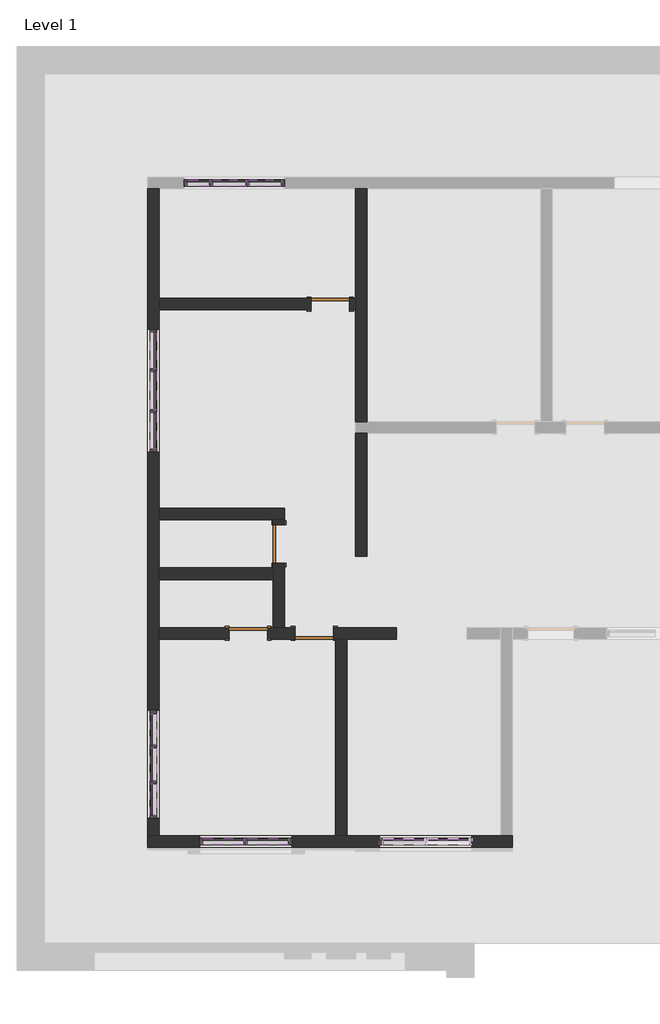
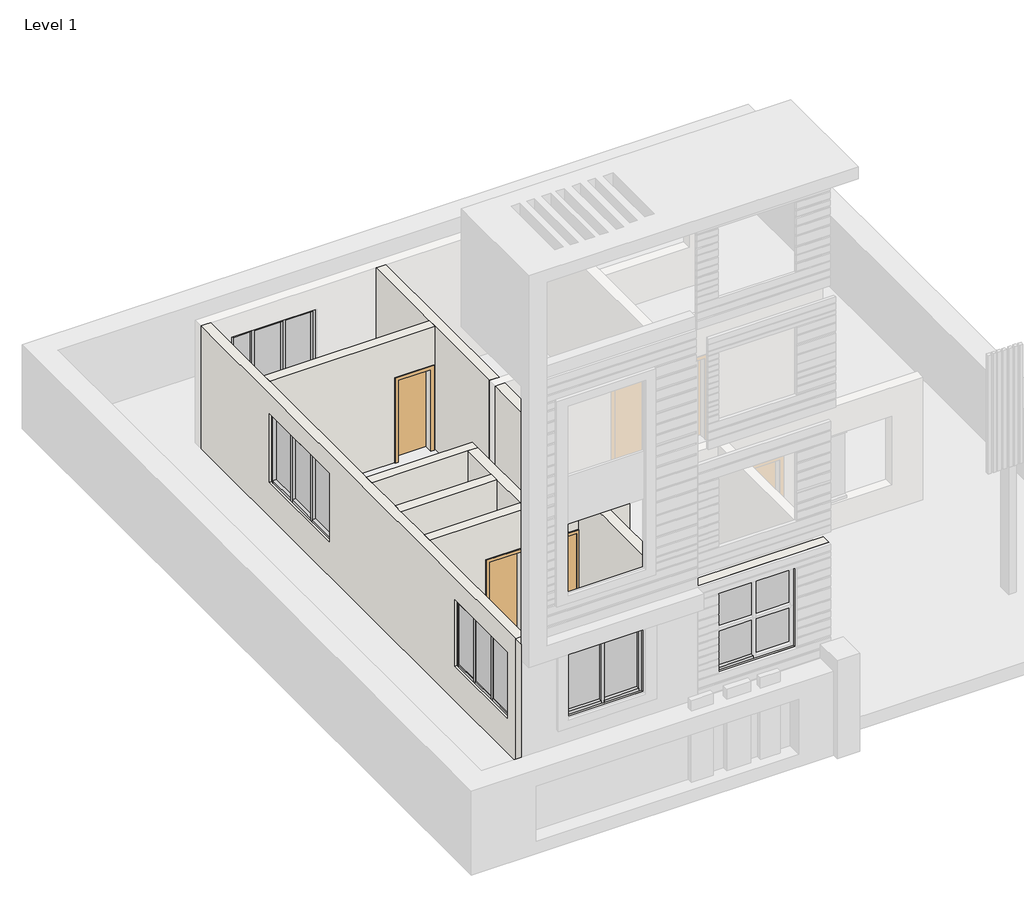
# One storey, part 1 of 2: 40 members, 15 plates, 10 walls, 4 doors.
"""IFC4 building model written with IfcOpenShell, lengths in millimetres."""

from ifc_helpers import new_model, si_unit, frame, origin, origin_with_axes, place, context, project, spatial, polyline, outline, extrude, faceted_brep, transform, mapped, element, save
from components import door_a1484949, door_85036156, member_3f0e0172, member_5215b92c, member_9d02be77, member_7007ad49, member_6fb4a552, member_d3852687, member_e7529cf5, member_eb14d2b7, member_dad99500, member_6c7e385d, member_4ab5fd4c, member_e2451291, member_36da3e1e, member_c17f1be2, member_e156fde9, member_8182dde8, member_6e7b816b, system_panel_glazed_5472c3c5, system_panel_glazed_33375d59, system_panel_glazed_3037aa96, system_panel_glazed_1cc22cd7, system_panel_glazed_f84acb07, system_panel_glazed_c72e3a3f, system_panel_glazed_c581bff3, system_panel_glazed_dab0583a, system_panel_glazed_6e362244

model = new_model("IFC4")

# Units and contexts
model_context = context("Model", 3, world=origin())
ifc_project = project(units=[si_unit("LENGTHUNIT", "METRE", prefix="MILLI")], contexts=[model_context])

# Site, building, storey
site = spatial("IfcSite", under=ifc_project)
building = spatial("IfcBuilding", under=site)
storey = spatial("IfcBuildingStorey", under=building, Name="Level 1", Elevation=0.0)

# Doors
placement = place(None, origin())
door_shape = door_a1484949(model_context)
element("IfcDoor", 1, ObjectType="Single-Flush : 30\" x 80\"", at=placement, inside=storey, context=model_context, shape_type="MappedRepresentation", body=[
    mapped(door_shape, transform((-16666.091855, -3109.9538163, 0.0), x_axis=(1.0, 0.0, 0.0), y_axis=(0.0, 1.0, 0.0), z_axis=(0.0, 0.0, 1.0))),
])
element("IfcDoor", 2, ObjectType="Single-Flush : 30\" x 80\"", at=placement, inside=storey, context=model_context, shape_type="MappedRepresentation", body=[
    mapped(door_shape, transform((-18291.691855, -9625.0538163, 0.0), x_axis=(1.0, 0.0, 0.0), y_axis=(0.0, 1.0, 0.0), z_axis=(0.0, 0.0, 1.0))),
])
door_2_shape = door_85036156(model_context)
element("IfcDoor", 3, ObjectType="Single-Flush : 30\" x 80\"", at=placement, inside=storey, context=model_context, shape_type="MappedRepresentation", body=[
    mapped(door_2_shape, transform((-16983.591855, -9625.0538163, 0.0), x_axis=(1.0, 0.0, 0.0), y_axis=(0.0, 1.0, 0.0), z_axis=(0.0, 0.0, 1.0))),
])
element("IfcDoor", 4, ObjectType="Single-Flush : 30\" x 80\"", at=placement, inside=storey, context=model_context, shape_type="MappedRepresentation", body=[
    mapped(door_2_shape, transform((-17682.091855, -7853.4038163, 0.0), x_axis=(0.0, -1.0, 0.0), y_axis=(1.0, 0.0, 0.0), z_axis=(0.0, 0.0, 1.0))),
])

# Members
member_shape = member_3f0e0172(model_context)
element("IfcMember", 5, ObjectType="Rectangular Mullion : 2.5\" x 5\" rectangular", at=placement, inside=storey, context=model_context, shape_type="MappedRepresentation", body=[
    mapped(member_shape, transform((-20171.291855, -11828.5038163, 858.7577978), x_axis=(0.0, 0.0, -1.0), y_axis=(1.0, 0.0, 0.0), z_axis=(0.0, -1.0, 0.0))),
])
element("IfcMember", 6, ObjectType="Rectangular Mullion : 2.5\" x 5\" rectangular", at=placement, inside=storey, context=model_context, shape_type="MappedRepresentation", body=[
    mapped(member_shape, transform((-20171.291855, -13219.1538163, 858.7577978), x_axis=(0.0, 0.0, -1.0), y_axis=(1.0, 0.0, 0.0), z_axis=(0.0, -1.0, 0.0))),
])
member_2_shape = member_5215b92c(model_context)
element("IfcMember", 7, ObjectType="Rectangular Mullion : 2.5\" x 5\" rectangular", at=placement, inside=storey, context=model_context, shape_type="MappedRepresentation", body=[
    mapped(member_2_shape, transform((-20171.291855, -12539.7038163, 858.7577978), x_axis=(0.0, 0.0, -1.0), y_axis=(1.0, 0.0, 0.0), z_axis=(0.0, -1.0, 0.0))),
])
element("IfcMember", 8, ObjectType="Rectangular Mullion : 2.5\" x 5\" rectangular", at=placement, inside=storey, context=model_context, shape_type="MappedRepresentation", body=[
    mapped(member_2_shape, transform((-20171.291855, -11892.0038163, 2504.227915), x_axis=(0.0, 0.0, 1.0), y_axis=(1.0, 0.0, 0.0), z_axis=(0.0, 1.0, 0.0))),
])
element("IfcMember", 9, ObjectType="Rectangular Mullion : 2.5\" x 5\" rectangular", at=placement, inside=storey, context=model_context, shape_type="MappedRepresentation", body=[
    mapped(member_shape, transform((-20171.291855, -12603.2038163, 2504.227915), x_axis=(0.0, 0.0, 1.0), y_axis=(1.0, 0.0, 0.0), z_axis=(0.0, 1.0, 0.0))),
])
element("IfcMember", 10, ObjectType="Rectangular Mullion : 2.5\" x 5\" rectangular", at=placement, inside=storey, context=model_context, shape_type="MappedRepresentation", body=[
    mapped(member_shape, transform((-20171.291855, -11212.5538163, 2504.227915), x_axis=(0.0, 0.0, 1.0), y_axis=(1.0, 0.0, 0.0), z_axis=(0.0, 1.0, 0.0))),
])
member_3_shape = member_9d02be77(model_context)
element("IfcMember", 11, ObjectType="Rectangular Mullion : 2.5\" x 5\" rectangular", at=placement, inside=storey, context=model_context, shape_type="MappedRepresentation", body=[
    mapped(member_3_shape, transform((-20171.291855, -4449.8038163, 849.1440376), x_axis=(0.0, 0.0, -1.0), y_axis=(-1.0, 0.0, 0.0), z_axis=(0.0, 1.0, 0.0))),
])
member_4_shape = member_7007ad49(model_context)
element("IfcMember", 12, ObjectType="Rectangular Mullion : 2.5\" x 5\" rectangular", at=placement, inside=storey, context=model_context, shape_type="MappedRepresentation", body=[
    mapped(member_4_shape, transform((-20171.291855, -5262.6038163, 849.1440376), x_axis=(0.0, 0.0, -1.0), y_axis=(-1.0, 0.0, 0.0), z_axis=(0.0, 1.0, 0.0))),
])
element("IfcMember", 13, ObjectType="Rectangular Mullion : 2.5\" x 5\" rectangular", at=placement, inside=storey, context=model_context, shape_type="MappedRepresentation", body=[
    mapped(member_4_shape, transform((-20171.291855, -3668.7538163, 849.1440376), x_axis=(0.0, 0.0, -1.0), y_axis=(-1.0, 0.0, 0.0), z_axis=(0.0, 1.0, 0.0))),
])
element("IfcMember", 14, ObjectType="Rectangular Mullion : 2.5\" x 5\" rectangular", at=placement, inside=storey, context=model_context, shape_type="MappedRepresentation", body=[
    mapped(member_4_shape, transform((-20171.291855, -4386.3038163, 2558.0352186), x_axis=(0.0, 0.0, 1.0), y_axis=(-1.0, 0.0, 0.0), z_axis=(0.0, -1.0, 0.0))),
])
element("IfcMember", 15, ObjectType="Rectangular Mullion : 2.5\" x 5\" rectangular", at=placement, inside=storey, context=model_context, shape_type="MappedRepresentation", body=[
    mapped(member_4_shape, transform((-20171.291855, -5980.1538163, 2558.0352186), x_axis=(0.0, 0.0, 1.0), y_axis=(-1.0, 0.0, 0.0), z_axis=(0.0, -1.0, 0.0))),
])
element("IfcMember", 16, ObjectType="Rectangular Mullion : 2.5\" x 5\" rectangular", at=placement, inside=storey, context=model_context, shape_type="MappedRepresentation", body=[
    mapped(member_3_shape, transform((-20171.291855, -5199.1038163, 2558.0352186), x_axis=(0.0, 0.0, 1.0), y_axis=(-1.0, 0.0, 0.0), z_axis=(0.0, -1.0, 0.0))),
])
member_5_shape = member_6fb4a552(model_context)
element("IfcMember", 17, ObjectType="Rectangular Mullion : 2.5\" x 5\" rectangular", at=placement, inside=storey, context=model_context, shape_type="MappedRepresentation", body=[
    mapped(member_5_shape, transform((-19060.041855, -709.6538163, 2512.1183195), x_axis=(0.0, 0.0, 1.0), y_axis=(0.0, -1.0, 0.0), z_axis=(1.0, 0.0, 0.0))),
])
member_6_shape = member_d3852687(model_context)
element("IfcMember", 18, ObjectType="Rectangular Mullion : 2.5\" x 5\" rectangular", at=placement, inside=storey, context=model_context, shape_type="MappedRepresentation", body=[
    mapped(member_6_shape, transform((-18336.141855, -709.6538163, 2512.1183195), x_axis=(0.0, 0.0, 1.0), y_axis=(0.0, -1.0, 0.0), z_axis=(1.0, 0.0, 0.0))),
])
member_7_shape = member_e7529cf5(model_context)
element("IfcMember", 19, ObjectType="Rectangular Mullion : 2.5\" x 5\" rectangular", at=placement, inside=storey, context=model_context, shape_type="MappedRepresentation", body=[
    mapped(member_7_shape, transform((-19028.291855, -709.6538163, 954.7607085), x_axis=(1.0, 0.0, 0.0), y_axis=(0.0, -1.0, 0.0), z_axis=(0.0, 0.0, -1.0))),
])
element("IfcMember", 20, ObjectType="Rectangular Mullion : 2.5\" x 5\" rectangular", at=placement, inside=storey, context=model_context, shape_type="MappedRepresentation", body=[
    mapped(member_7_shape, transform((-18304.391855, -709.6538163, 954.7607085), x_axis=(1.0, 0.0, 0.0), y_axis=(0.0, -1.0, 0.0), z_axis=(0.0, 0.0, -1.0))),
])
element("IfcMember", 21, ObjectType="Rectangular Mullion : 2.5\" x 5\" rectangular", at=placement, inside=storey, context=model_context, shape_type="MappedRepresentation", body=[
    mapped(member_6_shape, transform((-18996.541855, -709.6538163, 954.7607085), x_axis=(0.0, 0.0, -1.0), y_axis=(0.0, -1.0, 0.0), z_axis=(-1.0, 0.0, 0.0))),
])
element("IfcMember", 22, ObjectType="Rectangular Mullion : 2.5\" x 5\" rectangular", at=placement, inside=storey, context=model_context, shape_type="MappedRepresentation", body=[
    mapped(member_5_shape, transform((-19498.191855, -709.6538163, 954.7607085), x_axis=(0.0, 0.0, -1.0), y_axis=(0.0, -1.0, 0.0), z_axis=(-1.0, 0.0, 0.0))),
])
member_8_shape = member_eb14d2b7(model_context)
element("IfcMember", 23, ObjectType="Rectangular Mullion : 2.5\" x 5\" rectangular", at=placement, inside=storey, context=model_context, shape_type="MappedRepresentation", body=[
    mapped(member_8_shape, transform((-19561.691855, -709.6538163, 2512.1183195), x_axis=(-1.0, 0.0, 0.0), y_axis=(0.0, -1.0, 0.0), z_axis=(0.0, 0.0, 1.0))),
])
member_9_shape = member_dad99500(model_context)
element("IfcMember", 24, ObjectType="Rectangular Mullion : 2.5\" x 5\" rectangular", at=placement, inside=storey, context=model_context, shape_type="MappedRepresentation", body=[
    mapped(member_9_shape, transform((-17631.291855, -709.6538163, 2512.1183195), x_axis=(0.0, 0.0, 1.0), y_axis=(0.0, -1.0, 0.0), z_axis=(1.0, 0.0, 0.0))),
])
element("IfcMember", 25, ObjectType="Rectangular Mullion : 2.5\" x 5\" rectangular", at=placement, inside=storey, context=model_context, shape_type="MappedRepresentation", body=[
    mapped(member_9_shape, transform((-18272.641855, -709.6538163, 954.7607085), x_axis=(0.0, 0.0, -1.0), y_axis=(0.0, -1.0, 0.0), z_axis=(-1.0, 0.0, 0.0))),
])
element("IfcMember", 26, ObjectType="Rectangular Mullion : 2.5\" x 5\" rectangular", at=placement, inside=storey, context=model_context, shape_type="MappedRepresentation", body=[
    mapped(member_8_shape, transform((-17567.791855, -709.6538163, 954.7607085), x_axis=(1.0, 0.0, 0.0), y_axis=(0.0, -1.0, 0.0), z_axis=(0.0, 0.0, -1.0))),
])
member_10_shape = member_6c7e385d(model_context)
element("IfcMember", 27, ObjectType="Rectangular Mullion : 2.5\" x 5\" rectangular", at=placement, inside=storey, context=model_context, shape_type="MappedRepresentation", body=[
    mapped(member_10_shape, transform((-20171.291855, -4418.0538163, 849.1440376), x_axis=(0.0, -1.0, 0.0), y_axis=(-1.0, 0.0, 0.0), z_axis=(0.0, 0.0, -1.0))),
])
element("IfcMember", 28, ObjectType="Rectangular Mullion : 2.5\" x 5\" rectangular", at=placement, inside=storey, context=model_context, shape_type="MappedRepresentation", body=[
    mapped(member_10_shape, transform((-20171.291855, -5230.8538163, 849.1440376), x_axis=(0.0, -1.0, 0.0), y_axis=(-1.0, 0.0, 0.0), z_axis=(0.0, 0.0, -1.0))),
])
member_11_shape = member_4ab5fd4c(model_context)
element("IfcMember", 29, ObjectType="Rectangular Mullion : 2.5\" x 5\" rectangular", at=placement, inside=storey, context=model_context, shape_type="MappedRepresentation", body=[
    mapped(member_11_shape, transform((-20171.291855, -3605.2538163, 2558.0352186), x_axis=(0.0, 1.0, 0.0), y_axis=(-1.0, 0.0, 0.0), z_axis=(0.0, 0.0, 1.0))),
])
element("IfcMember", 30, ObjectType="Rectangular Mullion : 2.5\" x 5\" rectangular", at=placement, inside=storey, context=model_context, shape_type="MappedRepresentation", body=[
    mapped(member_11_shape, transform((-20171.291855, -6043.6538163, 849.1440376), x_axis=(0.0, -1.0, 0.0), y_axis=(-1.0, 0.0, 0.0), z_axis=(0.0, 0.0, -1.0))),
])
member_12_shape = member_e2451291(model_context)
element("IfcMember", 31, ObjectType="Rectangular Mullion : 2.5\" x 5\" rectangular", at=placement, inside=storey, context=model_context, shape_type="MappedRepresentation", body=[
    mapped(member_12_shape, transform((-20171.291855, -11860.2538163, 858.7577978), x_axis=(0.0, 1.0, 0.0), y_axis=(1.0, 0.0, 0.0), z_axis=(0.0, 0.0, -1.0))),
])
element("IfcMember", 32, ObjectType="Rectangular Mullion : 2.5\" x 5\" rectangular", at=placement, inside=storey, context=model_context, shape_type="MappedRepresentation", body=[
    mapped(member_12_shape, transform((-20171.291855, -12571.4538163, 858.7577978), x_axis=(0.0, 1.0, 0.0), y_axis=(1.0, 0.0, 0.0), z_axis=(0.0, 0.0, -1.0))),
])
member_13_shape = member_36da3e1e(model_context)
element("IfcMember", 33, ObjectType="Rectangular Mullion : 2.5\" x 5\" rectangular", at=placement, inside=storey, context=model_context, shape_type="MappedRepresentation", body=[
    mapped(member_13_shape, transform((-20171.291855, -13282.6538163, 2504.227915), x_axis=(0.0, -1.0, 0.0), y_axis=(1.0, 0.0, 0.0), z_axis=(0.0, 0.0, 1.0))),
])
element("IfcMember", 34, ObjectType="Rectangular Mullion : 2.5\" x 5\" rectangular", at=placement, inside=storey, context=model_context, shape_type="MappedRepresentation", body=[
    mapped(member_13_shape, transform((-20171.291855, -11149.0538163, 858.7577978), x_axis=(0.0, 1.0, 0.0), y_axis=(1.0, 0.0, 0.0), z_axis=(0.0, 0.0, -1.0))),
])
member_14_shape = member_c17f1be2(model_context)
element("IfcMember", 35, ObjectType="Rectangular Mullion : 2.5\" x 5\" rectangular", at=placement, inside=storey, context=model_context, shape_type="MappedRepresentation", body=[
    mapped(member_14_shape, transform((-18374.241855, -13739.8538163, 2645.3232141), x_axis=(0.0, 0.0, 1.0), y_axis=(0.0, -1.0, 0.0), z_axis=(1.0, 0.0, 0.0))),
])
element("IfcMember", 36, ObjectType="Rectangular Mullion : 2.5\" x 5\" rectangular", at=placement, inside=storey, context=model_context, shape_type="MappedRepresentation", body=[
    mapped(member_14_shape, transform((-17491.591855, -13739.8538163, 2645.3232141), x_axis=(0.0, 0.0, 1.0), y_axis=(0.0, -1.0, 0.0), z_axis=(1.0, 0.0, 0.0))),
])
member_15_shape = member_e156fde9(model_context)
element("IfcMember", 37, ObjectType="Rectangular Mullion : 2.5\" x 5\" rectangular", at=placement, inside=storey, context=model_context, shape_type="MappedRepresentation", body=[
    mapped(member_15_shape, transform((-15688.191855, -13739.8538163, 2743.3706019), x_axis=(-1.0, 0.0, 0.0), y_axis=(0.0, -1.0, 0.0), z_axis=(0.0, 0.0, 1.0))),
])
element("IfcMember", 38, ObjectType="Rectangular Mullion : 2.5\" x 5\" rectangular", at=placement, inside=storey, context=model_context, shape_type="MappedRepresentation", body=[
    mapped(member_14_shape, transform((-15624.691855, -13739.8538163, 741.3661492), x_axis=(0.0, 0.0, -1.0), y_axis=(0.0, -1.0, 0.0), z_axis=(-1.0, 0.0, 0.0))),
])
element("IfcMember", 39, ObjectType="Rectangular Mullion : 2.5\" x 5\" rectangular", at=placement, inside=storey, context=model_context, shape_type="MappedRepresentation", body=[
    mapped(member_14_shape, transform((-18310.741855, -13739.8538163, 874.5903603), x_axis=(0.0, 0.0, -1.0), y_axis=(0.0, -1.0, 0.0), z_axis=(-1.0, 0.0, 0.0))),
])
element("IfcMember", 40, ObjectType="Rectangular Mullion : 2.5\" x 5\" rectangular", at=placement, inside=storey, context=model_context, shape_type="MappedRepresentation", body=[
    mapped(member_14_shape, transform((-19193.391855, -13739.8538163, 874.5903603), x_axis=(0.0, 0.0, -1.0), y_axis=(0.0, -1.0, 0.0), z_axis=(-1.0, 0.0, 0.0))),
])
element("IfcMember", 41, ObjectType="Rectangular Mullion : 2.5\" x 5\" rectangular", at=placement, inside=storey, context=model_context, shape_type="MappedRepresentation", body=[
    mapped(member_15_shape, transform((-15688.191855, -13739.8538163, 1742.3683755), x_axis=(-1.0, 0.0, 0.0), y_axis=(0.0, -1.0, 0.0), z_axis=(0.0, 0.0, 1.0))),
])
member_16_shape = member_8182dde8(model_context)
element("IfcMember", 42, ObjectType="Rectangular Mullion : 2.5\" x 5\" rectangular", at=placement, inside=storey, context=model_context, shape_type="MappedRepresentation", body=[
    mapped(member_16_shape, transform((-18342.491855, -13739.8538163, 874.5903603), x_axis=(1.0, 0.0, 0.0), y_axis=(0.0, -1.0, 0.0), z_axis=(0.0, 0.0, -1.0))),
])
member_17_shape = member_6e7b816b(model_context)
element("IfcMember", 43, ObjectType="Rectangular Mullion : 2.5\" x 5\" rectangular", at=placement, inside=storey, context=model_context, shape_type="MappedRepresentation", body=[
    mapped(member_17_shape, transform((-17428.091855, -13739.8538163, 874.5903603), x_axis=(1.0, 0.0, 0.0), y_axis=(0.0, -1.0, 0.0), z_axis=(0.0, 0.0, -1.0))),
])
element("IfcMember", 44, ObjectType="Rectangular Mullion : 2.5\" x 5\" rectangular", at=placement, inside=storey, context=model_context, shape_type="MappedRepresentation", body=[
    mapped(member_17_shape, transform((-19256.891855, -13739.8538163, 2645.3232141), x_axis=(-1.0, 0.0, 0.0), y_axis=(0.0, -1.0, 0.0), z_axis=(0.0, 0.0, 1.0))),
])

# Plates
system_panel_glazed_shape = system_panel_glazed_5472c3c5(model_context)
element("IfcPlate", 45, ObjectType="System Panel : Glazed", at=placement, inside=storey, context=model_context, shape_type="MappedRepresentation", body=[
    mapped(system_panel_glazed_shape, transform((-19279.116855, -709.6538163, 1018.2607085), x_axis=(1.0, 0.0, 0.0), y_axis=(0.0, 1.0, 0.0), z_axis=(0.0, 0.0, 1.0))),
])
system_panel_glazed_2_shape = system_panel_glazed_33375d59(model_context)
element("IfcPlate", 46, ObjectType="System Panel : Glazed", at=placement, inside=storey, context=model_context, shape_type="MappedRepresentation", body=[
    mapped(system_panel_glazed_2_shape, transform((-18666.341855, -709.6538163, 1018.2607085), x_axis=(1.0, 0.0, 0.0), y_axis=(0.0, 1.0, 0.0), z_axis=(0.0, 0.0, 1.0))),
])
system_panel_glazed_3_shape = system_panel_glazed_3037aa96(model_context)
element("IfcPlate", 47, ObjectType="System Panel : Glazed", at=placement, inside=storey, context=model_context, shape_type="MappedRepresentation", body=[
    mapped(system_panel_glazed_3_shape, transform((-17951.966855, -709.6538163, 1018.2607085), x_axis=(1.0, 0.0, 0.0), y_axis=(0.0, 1.0, 0.0), z_axis=(0.0, 0.0, 1.0))),
])
system_panel_glazed_4_shape = system_panel_glazed_1cc22cd7(model_context)
element("IfcPlate", 48, ObjectType="System Panel : Glazed", at=placement, inside=storey, context=model_context, shape_type="MappedRepresentation", body=[
    mapped(system_panel_glazed_4_shape, transform((-20171.291855, -4027.5288163, 912.6440376), x_axis=(0.0, -1.0, 0.0), y_axis=(1.0, 0.0, 0.0), z_axis=(0.0, 0.0, 1.0))),
])
element("IfcPlate", 49, ObjectType="System Panel : Glazed", at=placement, inside=storey, context=model_context, shape_type="MappedRepresentation", body=[
    mapped(system_panel_glazed_4_shape, transform((-20171.291855, -5621.3788163, 912.6440376), x_axis=(0.0, -1.0, 0.0), y_axis=(1.0, 0.0, 0.0), z_axis=(0.0, 0.0, 1.0))),
])
system_panel_glazed_5_shape = system_panel_glazed_f84acb07(model_context)
element("IfcPlate", 50, ObjectType="System Panel : Glazed", at=placement, inside=storey, context=model_context, shape_type="MappedRepresentation", body=[
    mapped(system_panel_glazed_5_shape, transform((-20171.291855, -4824.4538163, 912.6440376), x_axis=(0.0, -1.0, 0.0), y_axis=(1.0, 0.0, 0.0), z_axis=(0.0, 0.0, 1.0))),
])
system_panel_glazed_6_shape = system_panel_glazed_c72e3a3f(model_context)
element("IfcPlate", 51, ObjectType="System Panel : Glazed", at=placement, inside=storey, context=model_context, shape_type="MappedRepresentation", body=[
    mapped(system_panel_glazed_6_shape, transform((-20171.291855, -12911.1788163, 922.2577978), x_axis=(0.0, 1.0, 0.0), y_axis=(-1.0, 0.0, 0.0), z_axis=(0.0, 0.0, 1.0))),
])
element("IfcPlate", 52, ObjectType="System Panel : Glazed", at=placement, inside=storey, context=model_context, shape_type="MappedRepresentation", body=[
    mapped(system_panel_glazed_6_shape, transform((-20171.291855, -11520.5288163, 922.2577978), x_axis=(0.0, 1.0, 0.0), y_axis=(-1.0, 0.0, 0.0), z_axis=(0.0, 0.0, 1.0))),
])
system_panel_glazed_7_shape = system_panel_glazed_c581bff3(model_context)
element("IfcPlate", 53, ObjectType="System Panel : Glazed", at=placement, inside=storey, context=model_context, shape_type="MappedRepresentation", body=[
    mapped(system_panel_glazed_7_shape, transform((-20171.291855, -12215.8538163, 922.2577978), x_axis=(0.0, 1.0, 0.0), y_axis=(-1.0, 0.0, 0.0), z_axis=(0.0, 0.0, 1.0))),
])
system_panel_glazed_8_shape = system_panel_glazed_dab0583a(model_context)
element("IfcPlate", 54, ObjectType="System Panel : Glazed", at=placement, inside=storey, context=model_context, shape_type="MappedRepresentation", body=[
    mapped(system_panel_glazed_8_shape, transform((-15215.116855, -13739.8538163, 804.8661492), x_axis=(1.0, 0.0, 0.0), y_axis=(0.0, 1.0, 0.0), z_axis=(0.0, 0.0, 1.0))),
])
element("IfcPlate", 55, ObjectType="System Panel : Glazed", at=placement, inside=storey, context=model_context, shape_type="MappedRepresentation", body=[
    mapped(system_panel_glazed_8_shape, transform((-14332.466855, -13739.8538163, 804.8661492), x_axis=(1.0, 0.0, 0.0), y_axis=(0.0, 1.0, 0.0), z_axis=(0.0, 0.0, 1.0))),
])
element("IfcPlate", 56, ObjectType="System Panel : Glazed", at=placement, inside=storey, context=model_context, shape_type="MappedRepresentation", body=[
    mapped(system_panel_glazed_8_shape, transform((-15215.116855, -13739.8538163, 1774.1183755), x_axis=(1.0, 0.0, 0.0), y_axis=(0.0, 1.0, 0.0), z_axis=(0.0, 0.0, 1.0))),
])
element("IfcPlate", 57, ObjectType="System Panel : Glazed", at=placement, inside=storey, context=model_context, shape_type="MappedRepresentation", body=[
    mapped(system_panel_glazed_8_shape, transform((-14332.466855, -13739.8538163, 1774.1183755), x_axis=(1.0, 0.0, 0.0), y_axis=(0.0, 1.0, 0.0), z_axis=(0.0, 0.0, 1.0))),
])
system_panel_glazed_9_shape = system_panel_glazed_6e362244(model_context)
element("IfcPlate", 58, ObjectType="System Panel : Glazed", at=placement, inside=storey, context=model_context, shape_type="MappedRepresentation", body=[
    mapped(system_panel_glazed_9_shape, transform((-18783.816855, -13739.8538163, 938.0903603), x_axis=(1.0, 0.0, 0.0), y_axis=(0.0, 1.0, 0.0), z_axis=(0.0, 0.0, 1.0))),
])
element("IfcPlate", 59, ObjectType="System Panel : Glazed", at=placement, inside=storey, context=model_context, shape_type="MappedRepresentation", body=[
    mapped(system_panel_glazed_9_shape, transform((-17901.166855, -13739.8538163, 938.0903603), x_axis=(1.0, 0.0, 0.0), y_axis=(0.0, 1.0, 0.0), z_axis=(0.0, 0.0, 1.0))),
])

# Walls
element("IfcWall", 60, ObjectType="9\"", at=placement, inside=storey, context=model_context, shape_type="Brep", body=[
    faceted_brep([(-20285.591855, -13854.1538163, 0.0), (-13059.291855, -13854.1538163, 0.0), (-13059.291855, -13854.1538163, 3048.0), (-20285.591855, -13854.1538163, 3048.0), (-15688.191855, -13854.1538163, 741.3661492), (-15688.191855, -13854.1538163, 2743.3706019), (-13859.391855, -13854.1538163, 2743.3706019), (-13859.391855, -13854.1538163, 741.3661492), (-19256.891855, -13854.1538163, 874.5903603), (-19256.891855, -13854.1538163, 2645.3232141), (-17428.091855, -13854.1538163, 2645.3232141), (-17428.091855, -13854.1538163, 874.5903603), (-13059.291855, -13625.5538163, 0.0), (-13287.891855, -13625.5538163, 0.0), (-16335.891855, -13625.5538163, 0.0), (-16564.491855, -13625.5538163, 0.0), (-20056.991855, -13625.5538163, 0.0), (-20285.591855, -13625.5538163, 0.0), (-20285.591855, -13625.5538163, 3048.0), (-20056.991855, -13625.5538163, 3048.0), (-16564.491855, -13625.5538163, 3048.0), (-16335.891855, -13625.5538163, 3048.0), (-13287.891855, -13625.5538163, 3048.0), (-13059.291855, -13625.5538163, 3048.0), (-15688.191855, -13625.5538163, 2743.3706019), (-15688.191855, -13625.5538163, 741.3661492), (-13859.391855, -13625.5538163, 741.3661492), (-13859.391855, -13625.5538163, 2743.3706019), (-19256.891855, -13625.5538163, 2645.3232141), (-19256.891855, -13625.5538163, 874.5903603), (-17428.091855, -13625.5538163, 874.5903603), (-17428.091855, -13625.5538163, 2645.3232141)], [[[0, 1, 2, 3], [4, 5, 6, 7], [8, 9, 10, 11]], [[12, 13, 14, 15, 16, 17, 18, 19, 20, 21, 22, 23], [24, 25, 26, 27], [28, 29, 30, 31]], [[1, 0, 17, 16, 15, 14, 13, 12]], [[2, 1, 12, 23]], [[3, 2, 23, 22, 21, 20, 19, 18]], [[0, 3, 18, 17]], [[24, 5, 4, 25]], [[5, 24, 27, 6]], [[6, 27, 26, 7]], [[25, 4, 7, 26]], [[8, 29, 28, 9]], [[9, 28, 31, 10]], [[10, 31, 30, 11]], [[29, 8, 11, 30]]]),
])
element("IfcWall", 61, ObjectType="9\"", at=placement, inside=storey, context=model_context, shape_type="Brep", body=[
    faceted_brep([(-20285.591855, -823.9538163, 0.0), (-20285.591855, -13625.5538163, 0.0), (-20285.591855, -13625.5538163, 3048.0), (-20285.591855, -823.9538163, 3048.0), (-20285.591855, -3605.2538163, 849.1440376), (-20285.591855, -3605.2538163, 2558.0352186), (-20285.591855, -6043.6538163, 2558.0352186), (-20285.591855, -6043.6538163, 849.1440376), (-20285.591855, -13282.6538163, 2504.227915), (-20285.591855, -13282.6538163, 858.7577978), (-20285.591855, -11149.0538163, 858.7577978), (-20285.591855, -11149.0538163, 2504.227915), (-20056.991855, -13625.5538163, 0.0), (-20056.991855, -9739.3538163, 0.0), (-20056.991855, -9510.7538163, 0.0), (-20056.991855, -8558.2538163, 0.0), (-20056.991855, -8329.6538163, 0.0), (-20056.991855, -7377.1538163, 0.0), (-20056.991855, -7148.5538163, 0.0), (-20056.991855, -3224.2538163, 0.0), (-20056.991855, -2995.6538163, 0.0), (-20056.991855, -823.9538163, 0.0), (-20056.991855, -823.9538163, 3048.0), (-20056.991855, -2995.6538163, 3048.0), (-20056.991855, -3224.2538163, 3048.0), (-20056.991855, -7148.5538163, 3048.0), (-20056.991855, -7377.1538163, 3048.0), (-20056.991855, -8329.6538163, 3048.0), (-20056.991855, -8558.2538163, 3048.0), (-20056.991855, -9510.7538163, 3048.0), (-20056.991855, -9739.3538163, 3048.0), (-20056.991855, -13625.5538163, 3048.0), (-20056.991855, -3605.2538163, 2558.0352186), (-20056.991855, -3605.2538163, 849.1440376), (-20056.991855, -6043.6538163, 849.1440376), (-20056.991855, -6043.6538163, 2558.0352186), (-20056.991855, -13282.6538163, 858.7577978), (-20056.991855, -13282.6538163, 2504.227915), (-20056.991855, -11149.0538163, 2504.227915), (-20056.991855, -11149.0538163, 858.7577978)], [[[0, 1, 2, 3], [4, 5, 6, 7], [8, 9, 10, 11]], [[12, 13, 14, 15, 16, 17, 18, 19, 20, 21, 22, 23, 24, 25, 26, 27, 28, 29, 30, 31], [32, 33, 34, 35], [36, 37, 38, 39]], [[1, 0, 21, 20, 19, 18, 17, 16, 15, 14, 13, 12]], [[3, 2, 31, 30, 29, 28, 27, 26, 25, 24, 23, 22]], [[0, 3, 22, 21]], [[2, 1, 12, 31]], [[32, 5, 4, 33]], [[5, 32, 35, 6]], [[6, 35, 34, 7]], [[33, 4, 7, 34]], [[36, 9, 8, 37]], [[37, 8, 11, 38]], [[38, 11, 10, 39]], [[9, 36, 39, 10]]]),
])
element("IfcWall", 62, ObjectType="9\"", at=placement, inside=storey, context=model_context, shape_type="SweptSolid", body=[
    extrude(outline(polyline([(-16335.891855, -9739.3538163), (-16335.891855, -13625.5538163), (-16564.491855, -13625.5538163), (-16564.491855, -9739.3538163), (-16335.891855, -9739.3538163)])), origin_with_axes(), (0.0, 0.0, 1.0), 3048.0),
])
element("IfcWall", 63, ObjectType="9\"", at=placement, inside=storey, context=model_context, shape_type="SweptSolid", body=[
    extrude(outline(polyline([(-17796.391855, -8558.2538163), (-20056.991855, -8558.2538163), (-20056.991855, -8329.6538163), (-17796.391855, -8329.6538163), (-17796.391855, -8558.2538163)])), origin_with_axes(), (0.0, 0.0, 1.0), 3048.0),
])
element("IfcWall", 64, ObjectType="9\"", at=placement, inside=storey, context=model_context, shape_type="Brep", body=[
    faceted_brep([(-17796.391855, -8234.4038163, 2032.0), (-17796.391855, -8234.4038163, 0.0), (-17796.391855, -8329.6538163, 0.0), (-17796.391855, -8558.2538163, 0.0), (-17796.391855, -9510.7538163, 0.0), (-17796.391855, -9510.7538163, 3048.0), (-17796.391855, -8558.2538163, 3048.0), (-17796.391855, -8329.6538163, 3048.0), (-17796.391855, -7377.1538163, 3048.0), (-17796.391855, -7377.1538163, 0.0), (-17796.391855, -7472.4038163, 0.0), (-17796.391855, -7472.4038163, 2032.0), (-17567.791855, -9510.7538163, 0.0), (-17567.791855, -8234.4038163, 0.0), (-17567.791855, -8234.4038163, 2032.0), (-17567.791855, -7472.4038163, 2032.0), (-17567.791855, -7472.4038163, 0.0), (-17567.791855, -7377.1538163, 0.0), (-17567.791855, -7377.1538163, 3048.0), (-17567.791855, -9510.7538163, 3048.0)], [[[0, 1, 2, 3, 4, 5, 6, 7, 8, 9, 10, 11]], [[12, 13, 14, 15, 16, 17, 18, 19]], [[10, 9, 17, 16]], [[4, 3, 2, 1, 13, 12]], [[8, 7, 6, 5, 19, 18]], [[5, 4, 12, 19]], [[9, 8, 18, 17]], [[14, 13, 1, 0]], [[15, 14, 0, 11]], [[16, 15, 11, 10]]]),
])
element("IfcWall", 65, ObjectType="9\"", at=placement, inside=storey, context=model_context, shape_type="Brep", body=[
    faceted_brep([(-20056.991855, -7377.1538163, 0.0), (-17796.391855, -7377.1538163, 0.0), (-17567.791855, -7377.1538163, 0.0), (-17567.791855, -7377.1538163, 3048.0), (-17796.391855, -7377.1538163, 3048.0), (-20056.991855, -7377.1538163, 3048.0), (-20056.991855, -7148.5538163, 0.0), (-20056.991855, -7148.5538163, 3048.0), (-17567.791855, -7148.5538163, 3048.0), (-17567.791855, -7148.5538163, 0.0)], [[[0, 1, 2, 3, 4, 5]], [[6, 7, 8, 9]], [[2, 1, 0, 6, 9]], [[5, 4, 3, 8, 7]], [[0, 5, 7, 6]], [[3, 2, 9, 8]]]),
])
element("IfcWall", 66, ObjectType="9\"", at=placement, inside=storey, context=model_context, shape_type="SweptSolid", body=[
    extrude(outline(polyline([(2032.0, -16285.091855), (0.0, -16285.091855), (0.0, -16170.791855), (3048.0, -16170.791855), (3048.0, -20056.991855), (0.0, -20056.991855), (0.0, -17047.091855), (2032.0, -17047.091855), (2032.0, -16285.091855)])), frame((0.0, -3224.2538163, 0.0), z_axis=(0.0, 1.0, 0.0), x_axis=(0.0, 0.0, 1.0)), (0.0, 0.0, 1.0), 228.6),
])
element("IfcWall", 67, ObjectType="9\"", at=placement, inside=storey, context=model_context, shape_type="SweptSolid", body=[
    extrude(outline(polyline([(-16170.791855, -8101.0538163), (-16170.791855, -5662.6538163), (-15942.191855, -5662.6538163), (-15942.191855, -8101.0538163), (-16170.791855, -8101.0538163)])), origin_with_axes(), (0.0, 0.0, 1.0), 3048.0),
])
element("IfcWall", 68, ObjectType="9\"", at=placement, inside=storey, context=model_context, shape_type="Brep", body=[
    faceted_brep([(-15942.191855, -5434.0538163, 0.0), (-15942.191855, -823.9538163, 0.0), (-15942.191855, -823.9538163, 3048.0), (-15942.191855, -5434.0538163, 3048.0), (-16170.791855, -5434.0538163, 0.0), (-16170.791855, -5434.0538163, 3048.0), (-16170.791855, -3224.2538163, 3048.0), (-16170.791855, -2995.6538163, 3048.0), (-16170.791855, -823.9538163, 3048.0), (-16170.791855, -823.9538163, 0.0), (-16170.791855, -2995.6538163, 0.0), (-16170.791855, -3224.2538163, 0.0)], [[[0, 1, 2, 3]], [[4, 5, 6, 7, 8, 9, 10, 11]], [[1, 0, 4, 11, 10, 9]], [[3, 2, 8, 7, 6, 5]], [[0, 3, 5, 4]], [[2, 1, 9, 8]]]),
])
element("IfcWall", 69, ObjectType="9\"", at=placement, inside=storey, context=model_context, shape_type="Brep", body=[
    faceted_brep([(-17364.591855, -9510.7538163, 0.0), (-17567.791855, -9510.7538163, 0.0), (-17796.391855, -9510.7538163, 0.0), (-17910.691855, -9510.7538163, 0.0), (-17910.691855, -9510.7538163, 2032.0), (-18672.691855, -9510.7538163, 2032.0), (-18672.691855, -9510.7538163, 0.0), (-20056.991855, -9510.7538163, 0.0), (-20056.991855, -9510.7538163, 3048.0), (-17796.391855, -9510.7538163, 3048.0), (-17567.791855, -9510.7538163, 3048.0), (-15357.991855, -9510.7538163, 3048.0), (-15357.991855, -9510.7538163, 0.0), (-16602.591855, -9510.7538163, 0.0), (-16602.591855, -9510.7538163, 2032.0), (-17364.591855, -9510.7538163, 2032.0), (-17910.691855, -9739.3538163, 2032.0), (-17910.691855, -9739.3538163, 0.0), (-17364.591855, -9739.3538163, 0.0), (-17364.591855, -9739.3538163, 2032.0), (-16602.591855, -9739.3538163, 2032.0), (-16602.591855, -9739.3538163, 0.0), (-16564.491855, -9739.3538163, 0.0), (-16335.891855, -9739.3538163, 0.0), (-15357.991855, -9739.3538163, 0.0), (-15357.991855, -9739.3538163, 3048.0), (-16335.891855, -9739.3538163, 3048.0), (-16564.491855, -9739.3538163, 3048.0), (-20056.991855, -9739.3538163, 3048.0), (-20056.991855, -9739.3538163, 0.0), (-18672.691855, -9739.3538163, 0.0), (-18672.691855, -9739.3538163, 2032.0)], [[[0, 1, 2, 3, 4, 5, 6, 7, 8, 9, 10, 11, 12, 13, 14, 15]], [[16, 17, 18, 19, 20, 21, 22, 23, 24, 25, 26, 27, 28, 29, 30, 31]], [[24, 23, 22, 21, 13, 12]], [[30, 29, 7, 6]], [[18, 17, 3, 2, 1, 0]], [[11, 10, 9, 8, 28, 27, 26, 25]], [[12, 11, 25, 24]], [[8, 7, 29, 28]], [[14, 13, 21, 20]], [[15, 14, 20, 19]], [[0, 15, 19, 18]], [[4, 3, 17, 16]], [[5, 4, 16, 31]], [[6, 5, 31, 30]]]),
])

save(model, "model.ifc")

# Revit data of these elements
# Type "Single-Flush : 30\" x 80\""
#   Type Mark = "5"
#   Construction Type Id = "MDOOR"
#   Assembly Code = "C1020"
#   Analytic Construction = "Metal"
#   Thickness = 0' - 2"
#   Heat Transfer Coefficient (U) = 0.651978 BTU/(h·ft²·°F)
#   Height = 6' - 8"
#   Trim Projection Ext = 0' - 1"
#   Trim Projection Int = 0' - 1"
#   Trim Width = 0' - 3"
#   Width = 2' - 6"
#   Define Thermal Properties by = 1
#   Define Thermal Properties by = 1
#   Door Material = Door - Panel
#   Frame Material = Door - Frame
#   Visual Light Transmittance = 0
#   Solar Heat Gain Coefficient = 0
#   Function = (empty or 0)
#   Wall Closure = (empty or 0)
# Type "Rectangular Mullion : 2.5\" x 5\" rectangular"
#   built-in parameter 1007304 = 0.416667 (stored number, unit not read)
#   built-in parameter 1007301 = 0.104167 (stored number, unit not read)
#   built-in parameter 1007300 = 0.104167 (stored number, unit not read)
# Type "System Panel : Glazed"
#   Construction Type Id = "GSP4R"
#   Analytic Construction = "1/8 in Pilkington single glazing"
#   Visual Light Transmittance = 0.9
#   Solar Heat Gain Coefficient = 0.86
#   Heat Transfer Coefficient (U) = 1.18115 BTU/(h·ft²·°F)
#   Define Thermal Properties by = 1
# Type "9\""
#   Assembly Code = "B2010"
#   Layers, outside or top first: 0' - 9" no material (function 1)
# Elements 1, 2, 3, 4 (IfcDoor, "Single-Flush : 30\" x 80\"")
#   Phase Created = New Construction
#   Materials on its faces: "Door - Frame", "Door - Panel"
# Elements 5, 6, 7, 8, 9, 10, 11, 12, 13, 14, 15, 16, 17, 18, 19, 20, 21, 22, 23, 24, 25, 26, 27, 28, 29, 30, 31, 32, 33, 34, 35, 36, 37, 38, 39, 40, 41, 42, 43, 44 (IfcMember, "Rectangular Mullion : 2.5\" x 5\" rectangular")
#   Phase Created = New Construction
#   Materials on its faces: "Aluminum"
# Elements 45, 46, 47, 48, 49, 50, 51, 52, 53, 54, 55, 56, 57, 58, 59 (IfcPlate, "System Panel : Glazed")
#   Phase Created = New Construction
#   Materials on its faces: "Glass"
# Elements 60, 61, 62, 63, 64, 65, 66, 67, 68, 69 (IfcWall, "9\"")
#   Top Offset = 0' - 0"
#   Base Offset = 0' - 0"
#   Unconnected Height = 10' - 0"
#   wall height = 10' - 0"
#   Phase Created = New Construction
#   Base Constraint = Level 1
#   Materials on its faces: "Default Wall"
# Materials
#   "Door - Panel": class "Wood", colour RGB 210 159 95, transparency 0, Cost = 0
#   "Door - Frame": colour RGB 118 70 51, transparency 0, Cost = 0
#   "Aluminum": class "Metal", colour RGB 247 247 247, transparency 0, Description = "Aluminum 6061", Cost = 0
#   "Glass": class "Glass", colour RGB 0 128 192, transparency 0.75, Description = "Soda Lime Glass", Cost = 0
#   "Default Wall": colour RGB 128 128 128, transparency 0, Cost = 0
